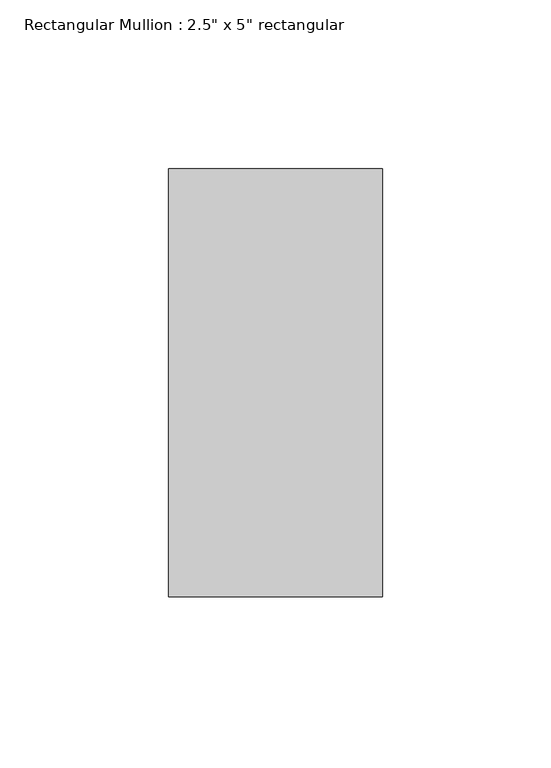
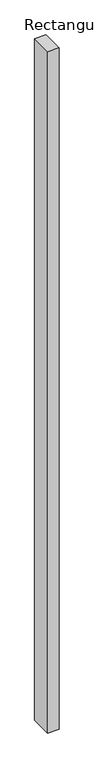
"""IFC4 building model written with IfcOpenShell, lengths in millimetres: member geometry."""

from ifc_helpers import new_model, si_unit, frame, origin, place, context, project, spatial, polyline, outline, extrude, source, transform, mapped, element, save


def member_9703a30f(model_context):
    return source(origin(), model_context, "Body", "SweptSolid", [
        extrude(outline(polyline([(0.0, 63.5), (0.0, -63.5), (-63.5, -63.5), (-63.5, 63.5), (0.0, 63.5)])), frame((0.0, 0.0, -4051.3), z_axis=(0.0, 0.0, 1.0), x_axis=(1.0, 0.0, 0.0)), (0.0, 0.0, 1.0), 4051.3),
    ])


if __name__ == "__main__":
    model = new_model("IFC4")
    model_context = context("Model", 3, world=origin())
    ifc_project = project(units=[si_unit("LENGTHUNIT", "METRE", prefix="MILLI")], contexts=[model_context])
    site = spatial("IfcSite", under=ifc_project)
    building = spatial("IfcBuilding", under=site)
    placement = place(None, origin())
    member_shape = member_9703a30f(model_context)
    element("IfcMember", 1, ObjectType="Rectangular Mullion : 2.5\" x 5\" rectangular", at=placement, inside=building, context=model_context, shape_type="MappedRepresentation", body=[
        mapped(member_shape, transform((0.0, 0.0, 0.0), x_axis=(1.0, 0.0, 0.0), y_axis=(0.0, 1.0, 0.0), z_axis=(0.0, 0.0, 1.0))),
    ])
    save(model, "model.ifc")

# Revit data of these elements
# Type "Rectangular Mullion : 2.5\" x 5\" rectangular"
#   built-in parameter 1007304 = 0.416667 (stored number, unit not read)
#   built-in parameter 1007301 = 0.104167 (stored number, unit not read)
#   built-in parameter 1007300 = 0.104167 (stored number, unit not read)
# Element 1 (IfcMember, "Rectangular Mullion : 2.5\" x 5\" rectangular")
#   Materials on its faces: "Iron, Ductile"
# Materials
#   "Iron, Ductile": class "Metal", colour RGB 0 0 0, transparency 0, Description = "Ductile cast iron", Cost = 0
